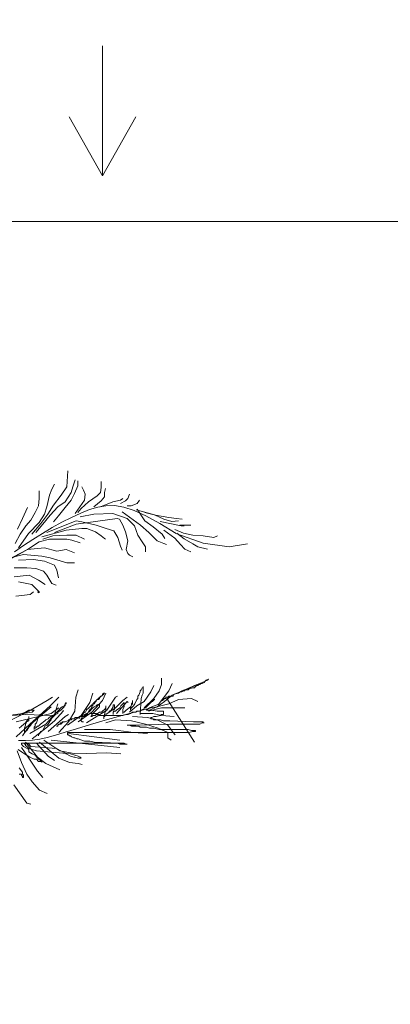
# Model space of a CAD drawing. Units: millimetres. Extents: x 595116 to 630915, y 909473 to 920225.
# Tile 40 of 134: x 629672 to 629682, y 919164 to 919190. Entities that reach past the tile are written whole.
import ezdxf

# ---------------------------------------------------------------- set-up
doc = ezdxf.new("R2010")
doc.units = ezdxf.units.MM
doc.layers.add('Dimension', color=3, linetype='Continuous', lineweight=18)
doc.layers.add('L-PLNT', color=85, linetype='Continuous', lineweight=13)
doc.styles.get("Standard").update_dxf_attribs({"font": 'arial.ttf'})
doc.dimstyles.new('ISO-25', dxfattribs={"dimtxt": 9, "dimasz": 6, "dimexe": 1.25, "dimexo": 0.625, "dimtad": 1, "dimlunit": 4, "dimtxsty": 'Standard', "dimcen": 2.5, "dimadec": 0, "dimazin": 0, "dimtfac": 1, "dimtmove": 0, "dimatfit": 3, "dimfxl": 1, "dimarcsym": 0})

# ---------------------------------------------------------------- blocks, each defined once
blk = doc.blocks.new('A$C4FB75ABC')
for p, q in [((4.1608, 3.5609), (4.1668, 3.6742)), ((4.2026, 3.5609), (4.2205, 3.6086)), ((4.2384, 3.5668), (4.2384, 3.6026)), ((4.4054, 3.5549), (4.4054, 3.5967)), ((3.964, 3.4774), (3.964, 3.5311)), ((4.0356, 3.5013), (4.0535, 3.543)), ((4.0535, 3.543), (4.0714, 3.5788)), ((4.1191, 3.5013), (4.1608, 3.5609)), ((4.1489, 3.4536), (4.1907, 3.5192)), ((4.1907, 3.5192), (4.2026, 3.5609)), ((4.1907, 3.4655), (4.2145, 3.5132)), ((4.2145, 3.5132), (4.2384, 3.5668)), ((4.2801, 3.537), (4.2682, 3.5609)), ((4.2921, 3.5072), (4.2801, 3.537)), ((4.3756, 3.4953), (4.3994, 3.5192)), ((4.3994, 3.5192), (4.4054, 3.5549)), ((4.4293, 3.5192), (4.4352, 3.549)), ((4.4293, 3.4893), (4.4293, 3.5192)), ((3.958, 3.4238), (3.964, 3.4774)), ((4.0177, 3.4178), (4.0356, 3.5013)), ((4.0654, 3.4297), (4.1191, 3.5013)), ((4.0952, 3.4178), (4.1489, 3.4536)), ((4.1489, 3.4118), (4.1907, 3.4655)), ((4.2205, 3.3701), (4.2861, 3.4655)), ((4.2622, 3.4059), (4.3159, 3.4536)), ((4.2861, 3.4655), (4.2921, 3.5072)), ((4.3159, 3.4536), (4.3756, 3.4953)), ((4.3517, 3.4178), (4.4054, 3.4595)), ((4.3994, 3.4178), (4.4889, 3.4536)), ((4.4054, 3.4595), (4.4293, 3.4893)), ((4.4889, 3.4536), (4.5426, 3.4655)), ((4.5426, 3.4655), (4.5605, 3.4774)), ((4.5426, 3.4416), (4.5784, 3.4595)), ((4.5784, 3.4595), (4.5963, 3.4774)), ((4.5963, 3.4774), (4.6082, 3.5072)), ((4.6619, 3.4416), (4.6798, 3.4655)), ((3.8447, 3.3343), (3.8805, 3.4118)), ((3.9044, 3.3224), (3.9342, 3.3761)), ((3.9342, 3.3761), (3.958, 3.4238)), ((3.9998, 3.3641), (4.0177, 3.4178)), ((4.0237, 3.3641), (4.0654, 3.4297)), ((4.0415, 3.3582), (4.0952, 3.4178)), ((4.1012, 3.3522), (4.1489, 3.4118)), ((4.1935, 3.342), (4.2593, 3.3722)), ((4.2384, 3.3761), (4.2622, 3.4059)), ((4.2593, 3.3722), (4.322, 3.3969)), ((4.322, 3.3969), (4.3813, 3.4152)), ((4.3813, 3.4152), (4.4396, 3.4254)), ((4.4396, 3.4254), (4.5001, 3.426)), ((4.5001, 3.426), (4.5657, 3.4153)), ((4.5545, 3.382), (4.6858, 3.2866)), ((4.5657, 3.4153), (4.6395, 3.3917)), ((4.5903, 3.4238), (4.6201, 3.4238)), ((4.6201, 3.4238), (4.6619, 3.4416)), ((4.6395, 3.3917), (4.7247, 3.3534)), ((4.6551, 3.396), (4.7847, 3.3597)), ((4.6619, 3.3999), (4.7156, 3.3164)), ((4.7156, 3.3761), (4.7931, 3.3582)), ((3.8089, 3.2568), (3.8447, 3.3343)), ((3.8686, 3.2807), (3.9044, 3.3224)), ((3.8865, 3.227), (3.964, 3.3045)), ((3.964, 3.3045), (3.9998, 3.3641)), ((3.9759, 3.2986), (4.0237, 3.3641)), ((3.9879, 3.2926), (4.0415, 3.3582)), ((4.0177, 3.233), (4.2265, 3.3164)), ((4.0565, 3.2687), (4.1256, 3.3072)), ((4.0654, 3.3105), (4.1012, 3.3522)), ((4.1256, 3.3072), (4.1935, 3.342)), ((4.2265, 3.2926), (4.5187, 3.3343)), ((4.2265, 3.3164), (4.2682, 3.3105)), ((4.2563, 3.3463), (4.3517, 3.3641)), ((4.2682, 3.3105), (4.3696, 3.2866)), ((4.3517, 3.3641), (4.4889, 3.3701)), ((4.4889, 3.3701), (4.5903, 3.3343)), ((4.5187, 3.3343), (4.5366, 3.3284)), ((4.5366, 3.3284), (4.5605, 3.2866)), ((4.5903, 3.3343), (4.644, 3.2807)), ((4.7156, 3.3164), (4.7752, 3.2747)), ((4.7247, 3.3534), (4.8242, 3.2989)), ((4.7847, 3.3597), (4.8521, 3.3286)), ((4.7931, 3.3582), (4.8886, 3.3403)), ((4.8262, 3.3131), (4.9765, 3.282)), ((4.8521, 3.3286), (4.9091, 3.3131)), ((4.8886, 3.3403), (4.9422, 3.3343)), ((4.9091, 3.3131), (4.9558, 3.3183)), ((4.9422, 3.3343), (4.984, 3.3284)), ((3.8268, 3.2211), (3.8686, 3.2807)), ((3.9103, 3.2211), (3.9759, 3.2986)), ((3.9401, 3.233), (3.9879, 3.2926)), ((3.9819, 3.2032), (4.1549, 3.2509)), ((3.9871, 3.2274), (4.0565, 3.2687)), ((4.0714, 3.233), (4.2265, 3.2926)), ((4.1549, 3.2509), (4.2682, 3.2628)), ((4.2682, 3.2628), (4.304, 3.2628)), ((4.304, 3.2628), (4.3637, 3.2389)), ((4.3637, 3.2389), (4.4054, 3.2091)), ((4.3696, 3.2866), (4.4412, 3.2628)), ((4.4412, 3.2628), (4.4949, 3.2449)), ((4.4949, 3.2449), (4.5247, 3.1972)), ((4.5605, 3.2866), (4.5784, 3.2389)), ((4.5784, 3.2389), (4.5963, 3.1734)), ((4.644, 3.2807), (4.6679, 3.2151)), ((4.6858, 3.2866), (4.7454, 3.233)), ((4.7454, 3.233), (4.8051, 3.1734)), ((4.7752, 3.2747), (4.8408, 3.2211)), ((4.8242, 3.2989), (4.9411, 3.2265)), ((4.8521, 3.2509), (4.9299, 3.1939)), ((4.9299, 3.2561), (4.9921, 3.2302)), ((4.9661, 3.2866), (5.0079, 3.2866)), ((4.9765, 3.282), (4.9973, 3.282)), ((5.0079, 3.2866), (5.0437, 3.2866)), ((3.791, 3.1555), (3.8268, 3.2211)), ((3.8149, 3.1257), (3.8865, 3.227)), ((3.8516, 3.1401), (3.9185, 3.1843)), ((3.8805, 3.1137), (3.964, 3.1674)), ((3.9185, 3.1843), (3.9871, 3.2274)), ((3.964, 3.1674), (4.0356, 3.1853)), ((3.9879, 3.1853), (4.0594, 3.2091)), ((4.0356, 3.1853), (4.1072, 3.1853)), ((4.0594, 3.2091), (4.1608, 3.2151)), ((4.1072, 3.1853), (4.1608, 3.1853)), ((4.1608, 3.2151), (4.2265, 3.2151)), ((4.1608, 3.1853), (4.1966, 3.1793)), ((4.1966, 3.1793), (4.2563, 3.1614)), ((4.2265, 3.2151), (4.2861, 3.1853)), ((4.4054, 3.2091), (4.4293, 3.1912)), ((4.4293, 3.1912), (4.4352, 3.1853)), ((4.5247, 3.1972), (4.5426, 3.1376)), ((4.5963, 3.1734), (4.5844, 3.1137)), ((4.6679, 3.2151), (4.6977, 3.1674)), ((4.6977, 3.1674), (4.7215, 3.1316)), ((4.8051, 3.1734), (4.8528, 3.1555)), ((4.8408, 3.2211), (4.8587, 3.1912)), ((4.9299, 3.1939), (4.9713, 3.1472)), ((4.9454, 3.2302), (4.9973, 3.1887)), ((4.9454, 3.225), (5.1321, 3.1576)), ((4.9921, 3.2302), (5.0595, 3.2146)), ((4.9973, 3.1887), (5.0595, 3.1524)), ((5.0595, 3.2146), (5.1321, 3.2094)), ((5.1321, 3.2094), (5.2099, 3.1991)), ((5.2099, 3.1991), (5.2358, 3.2094)), ((3.7433, 3.0362), (3.8805, 3.1137)), ((3.7791, 3.0601), (3.8805, 3.1137)), ((3.7873, 3.0958), (3.8516, 3.1401)), ((3.8805, 3.1137), (3.9998, 3.1257)), ((3.9998, 3.1257), (4.0893, 3.1018)), ((4.0893, 3.1018), (4.1549, 3.1137)), ((4.1549, 3.1137), (4.2145, 3.0899)), ((4.5426, 3.1376), (4.5545, 3.1078)), ((4.5844, 3.1137), (4.5963, 3.0839)), ((4.7215, 3.1316), (4.7215, 3.0959)), ((4.8528, 3.1555), (4.8707, 3.1495)), ((4.9713, 3.1472), (5.0025, 3.1162)), ((5.0025, 3.1162), (5.0439, 3.0954)), ((5.0595, 3.1524), (5.0958, 3.1317)), ((5.0958, 3.1317), (5.1632, 3.1162)), ((5.1321, 3.1576), (5.3187, 3.1317)), ((5.3187, 3.1317), (5.4484, 3.1524)), ((3.7552, 3.0541), (3.8507, 3.078)), ((3.8149, 3.0362), (3.9222, 3.0422)), ((3.8507, 3.078), (3.9819, 3.066)), ((3.9222, 3.0422), (3.9998, 3.0303)), ((3.9819, 3.066), (4.0415, 3.0541)), ((3.9998, 3.0303), (4.0714, 3.0005)), ((4.0415, 3.0541), (4.1608, 3.0184)), ((4.5963, 3.0839), (4.6082, 3.072)), ((4.6082, 3.072), (4.6321, 3.0601)), ((3.7851, 2.9826), (3.8745, 2.9826)), ((3.8745, 2.9826), (3.9401, 2.9766)), ((3.9401, 2.9766), (3.9938, 2.9587)), ((3.9938, 2.9587), (4.0177, 2.9289)), ((4.0714, 3.0005), (4.0893, 2.9647)), ((4.0893, 2.9647), (4.1012, 2.911)), ((4.1608, 3.0184), (4.2145, 3.0184)), ((3.7851, 2.917), (3.8924, 2.9289)), ((3.8149, 2.8812), (3.9103, 2.8633)), ((3.8924, 2.9289), (3.958, 2.8932)), ((3.958, 2.8932), (4.0058, 2.8633)), ((4.0177, 2.9289), (4.0535, 2.8693)), ((3.9103, 2.8633), (3.964, 2.8097)), ((4.0535, 2.8693), (4.0833, 2.8574)), ((3.797, 2.7799), (3.8984, 2.7918)), ((3.8984, 2.7918), (3.9222, 2.8097)), ((3.964, 2.8037), (3.9521, 2.8097)), ((3.964, 2.8097), (3.964, 2.8037)), ((4.835, 2.1495), (4.835, 2.1952)), ((5.1477, 2.1724), (5.1629, 2.18)), ((5.1553, 2.18), (5.1477, 2.1724)), ((5.1706, 2.1876), (5.1553, 2.18)), ((5.1629, 2.18), (5.1706, 2.1876)), ((4.2249, 2.058), (4.2402, 2.1114)), ((4.6825, 2.1038), (4.6901, 2.1114)), ((4.6901, 2.1114), (4.6977, 2.1266)), ((4.6977, 2.1266), (4.7054, 2.1266)), ((4.7054, 2.1266), (4.7054, 2.1343)), ((4.7054, 2.1343), (4.7054, 2.0885)), ((4.7587, 2.0961), (4.7816, 2.1419)), ((4.8198, 2.1038), (4.835, 2.1495)), ((4.8884, 2.1038), (4.9113, 2.1571)), ((4.9113, 2.0733), (5.079, 2.1419)), ((5.018, 2.119), (4.9799, 2.1038)), ((5.0028, 2.1038), (5.0028, 2.1114)), ((5.0028, 2.1114), (5.0257, 2.1114)), ((5.0333, 2.1266), (5.018, 2.119)), ((5.0257, 2.1114), (5.0333, 2.119)), ((5.0562, 2.1343), (5.0333, 2.1266)), ((5.0333, 2.119), (5.0562, 2.1266)), ((5.0714, 2.1419), (5.0562, 2.1343)), ((5.0562, 2.1266), (5.0714, 2.1266)), ((5.1095, 2.1571), (5.0714, 2.1419)), ((5.0714, 2.1266), (5.079, 2.1343)), ((5.079, 2.1343), (5.0867, 2.1419)), ((5.0867, 2.1419), (5.0943, 2.1419)), ((5.0943, 2.1419), (5.1019, 2.1495)), ((5.1019, 2.1495), (5.1095, 2.1495)), ((5.1248, 2.1648), (5.1095, 2.1571)), ((5.1095, 2.1495), (5.1172, 2.1571)), ((5.1172, 2.1571), (5.1248, 2.1571)), ((5.1477, 2.1724), (5.1248, 2.1648)), ((5.1248, 2.1571), (5.1401, 2.1648)), ((5.1401, 2.1648), (5.1477, 2.1724)), ((4.019, 2.0352), (4.0571, 2.058)), ((4.0419, 1.9971), (4.1029, 2.058)), ((4.2173, 1.9589), (4.2249, 2.058)), ((4.324, 2.0199), (4.3469, 2.0885)), ((4.3698, 2.0352), (4.3774, 2.0428)), ((4.3774, 2.0428), (4.3698, 2.0352)), ((4.3851, 2.0504), (4.3774, 2.0428)), ((4.3774, 2.0428), (4.3851, 2.0428)), ((4.3927, 2.058), (4.3851, 2.0504)), ((4.3851, 2.0428), (4.3927, 2.0504)), ((4.4079, 2.0657), (4.3927, 2.058)), ((4.3927, 2.0504), (4.3927, 2.058)), ((4.3927, 2.058), (4.4003, 2.058)), ((4.4003, 2.058), (4.4003, 2.0657)), ((4.4003, 2.0657), (4.4079, 2.0657)), ((4.4079, 2.0657), (4.4156, 2.0733)), ((4.4156, 2.0733), (4.4079, 2.0657)), ((4.4156, 2.0809), (4.4232, 2.0885)), ((4.4156, 2.0352), (4.4384, 2.0885)), ((4.4156, 2.0733), (4.4156, 2.0809)), ((4.4232, 2.0809), (4.4156, 2.0733)), ((4.4232, 2.0885), (4.4308, 2.0885)), ((4.4308, 2.0885), (4.4232, 2.0885)), ((4.4232, 2.0885), (4.4232, 2.0809)), ((4.4461, 1.9666), (4.5071, 2.058)), ((4.5071, 2.058), (4.5223, 2.0657)), ((4.5605, 2.0352), (4.591, 2.058)), ((4.6444, 2.0123), (4.6596, 2.0428)), ((4.6596, 2.0428), (4.6672, 2.0504)), ((4.6672, 2.0657), (4.6749, 2.0733)), ((4.6672, 2.0504), (4.6672, 2.0657)), ((4.6749, 2.0733), (4.6825, 2.0961)), ((4.6825, 2.0961), (4.6825, 2.1038)), ((4.6901, 2.0504), (4.6825, 1.9361)), ((4.6977, 2.0733), (4.6901, 2.0504)), ((4.7054, 2.0885), (4.6977, 2.0733)), ((4.713, 2.0275), (4.7587, 2.0961)), ((4.713, 1.9818), (4.7816, 2.0504)), ((4.7816, 2.0504), (4.8198, 2.1038)), ((4.7892, 2.0428), (4.7816, 2.0428)), ((4.7816, 2.0428), (4.7816, 2.0352)), ((4.8121, 2.0047), (4.8884, 2.1038)), ((4.8426, 2.0352), (4.8579, 2.0504)), ((4.8579, 2.0275), (4.9113, 2.0733)), ((4.8579, 2.0504), (4.8655, 2.0504)), ((4.8655, 2.0504), (4.8655, 2.058)), ((4.8655, 2.058), (4.8808, 2.058)), ((4.8808, 2.0504), (4.8731, 2.0504)), ((4.8731, 2.0504), (5.0714, 1.7379)), ((4.8808, 2.058), (4.8884, 2.0657)), ((4.896, 2.058), (4.8808, 2.058)), ((4.8808, 2.058), (4.8808, 2.0504)), ((4.8884, 2.0657), (4.9036, 2.0657)), ((4.8884, 2.0123), (4.957, 2.0428)), ((4.9036, 2.0657), (4.896, 2.058)), ((4.9036, 2.0657), (4.9113, 2.0733)), ((4.9189, 2.0657), (4.9036, 2.0657)), ((4.9113, 2.0733), (4.9265, 2.0809)), ((4.9265, 2.0809), (4.9189, 2.0657)), ((4.9265, 2.0809), (4.957, 2.0885)), ((4.9494, 2.0885), (4.9265, 2.0809)), ((4.9799, 2.1038), (4.9494, 2.0885)), ((4.957, 2.0885), (4.9723, 2.0961)), ((4.957, 2.0428), (5.0485, 2.0504)), ((4.9723, 2.0961), (4.9799, 2.0961)), ((4.9799, 2.0961), (4.9952, 2.1038)), ((4.9952, 2.1038), (5.0028, 2.1038)), ((5.0485, 2.0504), (5.0943, 2.0275)), ((3.8894, 1.9589), (4.019, 2.0352)), ((3.958, 1.9132), (4.0495, 1.9894)), ((3.9656, 1.9285), (4.0419, 1.9971)), ((4.0495, 1.9437), (4.1029, 1.9818)), ((4.0724, 1.9361), (4.0953, 2.0123)), ((4.1181, 1.9818), (4.1029, 1.9666)), ((4.1258, 1.9894), (4.1181, 1.9818)), ((4.1181, 1.9666), (4.1334, 1.9818)), ((4.141, 1.9971), (4.1258, 1.9894)), ((4.1334, 1.9818), (4.141, 1.9894)), ((4.1486, 2.0123), (4.141, 1.9971)), ((4.141, 1.9894), (4.141, 1.9971)), ((4.141, 1.9971), (4.1486, 1.9971)), ((4.1563, 2.0199), (4.1486, 2.0123)), ((4.1486, 1.9971), (4.1486, 2.0123)), ((4.1486, 2.0123), (4.1563, 2.0123)), ((4.1563, 2.0123), (4.1563, 2.0199)), ((4.263, 1.9285), (4.324, 2.0199)), ((4.3088, 1.9742), (4.3012, 1.9742)), ((4.3012, 1.9742), (4.3012, 1.9666)), ((4.3164, 1.9818), (4.3088, 1.9742)), ((4.3317, 1.9971), (4.3164, 1.9818)), ((4.3164, 1.9513), (4.3469, 1.9818)), ((4.324, 1.9666), (4.324, 1.9742)), ((4.324, 1.9742), (4.3317, 1.9742)), ((4.3393, 2.0047), (4.3317, 1.9971)), ((4.3317, 1.9742), (4.3393, 1.9894)), ((4.3393, 1.9513), (4.4156, 2.0352)), ((4.3546, 2.0123), (4.3393, 2.0047)), ((4.3393, 1.9894), (4.3393, 1.9971)), ((4.3393, 1.9971), (4.3469, 1.9971)), ((4.3469, 2.0123), (4.3622, 2.0275)), ((4.3469, 1.9971), (4.3469, 2.0123)), ((4.3469, 1.9818), (4.3546, 1.9894)), ((4.3698, 2.0352), (4.3546, 2.0123)), ((4.3546, 1.9894), (4.3698, 1.9971)), ((4.3622, 2.0275), (4.3698, 2.0275)), ((4.3698, 2.0275), (4.3698, 2.0352)), ((4.3698, 1.9971), (4.3774, 2.0047)), ((4.3851, 1.9818), (4.3698, 1.9666)), ((4.3774, 2.0047), (4.3927, 2.0123)), ((4.3927, 1.9894), (4.3851, 1.9818)), ((4.3927, 2.0123), (4.3927, 1.9894)), ((4.4156, 1.9589), (4.4308, 1.9742)), ((4.4308, 1.9742), (4.4384, 1.9818)), ((4.4384, 1.9818), (4.4384, 1.9971)), ((4.4384, 1.9971), (4.4384, 1.9589)), ((4.4384, 1.9361), (4.5071, 1.9818)), ((4.4766, 1.9666), (4.4918, 1.9894)), ((4.4918, 1.9894), (4.4918, 2.0047)), ((4.4918, 2.0047), (4.4995, 2.0047)), ((4.4995, 1.9742), (4.4918, 1.9513)), ((4.4995, 2.0047), (4.4995, 1.9742)), ((4.5071, 1.9818), (4.5605, 2.0352)), ((4.5147, 1.9437), (4.591, 2.0275)), ((4.5147, 1.9666), (4.5376, 1.9818)), ((4.5376, 1.9818), (4.5452, 1.9971)), ((4.5452, 1.9971), (4.5528, 2.0047)), ((4.5528, 2.0047), (4.5605, 2.0123)), ((4.5605, 2.0123), (4.5681, 2.0199)), ((4.5681, 1.9894), (4.5605, 1.9742)), ((4.5605, 1.9742), (4.5605, 1.9437)), ((4.5681, 2.0199), (4.5681, 1.9894)), ((4.5833, 1.9666), (4.6138, 1.9894)), ((4.591, 2.0275), (4.5986, 2.0199)), ((4.7725, 1.9851), (4.5975, 1.9398)), ((4.6062, 1.9513), (4.6596, 1.9971)), ((4.6138, 1.9894), (4.6215, 2.0047)), ((4.6215, 2.0047), (4.6138, 1.9818)), ((4.6138, 1.9818), (4.6138, 1.9666)), ((4.6138, 1.9742), (4.6215, 1.9818)), ((4.6138, 1.9666), (4.6138, 1.9742)), ((4.6215, 2.0123), (4.6291, 2.0199)), ((4.6215, 2.0047), (4.6215, 2.0123)), ((4.6291, 2.0123), (4.6215, 2.0047)), ((4.6215, 1.9818), (4.6367, 1.9971)), ((4.6291, 2.0199), (4.6291, 2.0352)), ((4.6291, 2.0352), (4.6291, 2.0123)), ((4.6367, 1.9971), (4.6444, 2.0123)), ((4.6596, 1.9971), (4.713, 2.0275)), ((4.7054, 1.9742), (4.6901, 1.9666)), ((4.7206, 1.9818), (4.7054, 1.9742)), ((4.7359, 1.9971), (4.7206, 1.9818)), ((4.7282, 1.9666), (4.7282, 1.9742)), ((4.7282, 1.9742), (4.7359, 1.9742)), ((4.7435, 2.0047), (4.7359, 1.9971)), ((4.7359, 1.9742), (4.7511, 1.9818)), ((4.7511, 2.0123), (4.7435, 2.0047)), ((4.7435, 1.9589), (4.835, 1.9818)), ((4.7664, 2.0275), (4.7511, 2.0123)), ((4.7511, 1.9818), (4.7664, 1.9894)), ((4.7511, 1.9666), (4.8045, 1.9894)), ((4.774, 2.0275), (4.7664, 2.0275)), ((4.7664, 1.9894), (4.8045, 2.0047)), ((4.7816, 2.0352), (4.774, 2.0352)), ((4.774, 2.0352), (4.774, 2.0275)), ((4.774, 1.9818), (4.8884, 2.0123)), ((4.8045, 1.9894), (4.8579, 2.0275)), ((4.8045, 2.0047), (4.8198, 2.0123)), ((4.8198, 2.0123), (4.8274, 2.0275)), ((4.8274, 2.0275), (4.8426, 2.0352)), ((4.835, 1.9818), (4.9494, 1.9818)), ((4.9494, 1.9818), (5.0028, 1.9818)), ((3.5843, 1.9132), (3.8665, 1.9361)), ((3.7445, 1.9285), (3.9122, 1.9513)), ((3.7521, 1.8903), (3.8894, 1.9589)), ((3.7978, 1.8827), (4.0495, 1.9437)), ((3.8665, 1.9513), (3.8207, 1.9361)), ((3.8894, 1.9666), (3.8665, 1.9513)), ((3.8665, 1.9361), (4.0495, 1.9285)), ((3.8894, 1.9056), (3.8741, 1.8903)), ((3.9275, 1.9666), (3.8894, 1.9666)), ((3.8894, 1.8903), (3.8894, 1.9208)), ((3.8894, 1.9208), (3.8894, 1.9056)), ((3.897, 1.8675), (3.9656, 1.9285)), ((3.897, 1.8599), (3.958, 1.9132)), ((3.9122, 1.9513), (3.9199, 1.9589)), ((3.9351, 1.898), (3.9122, 1.8751)), ((3.9199, 1.9589), (3.9275, 1.9666)), ((3.9504, 1.9056), (3.9351, 1.898)), ((3.9427, 1.8751), (3.9504, 1.898)), ((3.958, 1.9208), (3.9504, 1.9056)), ((3.9504, 1.9056), (3.958, 1.9132)), ((3.9504, 1.898), (3.9504, 1.9056)), ((3.958, 1.9208), (3.9656, 1.9285)), ((3.9656, 1.9285), (3.958, 1.9208)), ((3.958, 1.9132), (3.958, 1.9208)), ((3.9656, 1.9285), (3.9656, 1.9361)), ((3.9656, 1.9361), (3.9656, 1.9285)), ((4.0114, 1.898), (4.0037, 1.8903)), ((4.0114, 1.8675), (4.0724, 1.9361)), ((4.0266, 1.9056), (4.0114, 1.898)), ((4.0266, 1.8141), (4.1486, 1.9208)), ((4.0343, 1.9132), (4.0266, 1.9056)), ((4.0571, 1.9285), (4.0343, 1.9132)), ((4.0419, 1.8903), (4.0495, 1.898)), ((4.0495, 1.9056), (4.0571, 1.9132)), ((4.0495, 1.898), (4.0495, 1.9056)), ((4.0724, 1.9361), (4.0571, 1.9285)), ((4.0571, 1.9132), (4.0724, 1.9285)), ((4.0724, 1.8903), (4.1334, 1.9589)), ((4.08, 1.9437), (4.0724, 1.9361)), ((4.0724, 1.9285), (4.08, 1.9361)), ((4.1029, 1.9666), (4.08, 1.9437)), ((4.08, 1.9361), (4.0953, 1.9437)), ((4.0953, 1.9513), (4.1181, 1.9666)), ((4.0953, 1.9437), (4.0953, 1.9513)), ((4.1334, 1.9589), (4.1334, 1.9666)), ((4.1486, 1.9208), (4.1715, 1.9361)), ((4.1639, 1.8599), (4.263, 1.9285)), ((4.1715, 1.8827), (4.2173, 1.9589)), ((4.1944, 1.898), (4.1715, 1.898)), ((4.1715, 1.898), (4.1715, 1.8903)), ((4.2173, 1.9056), (4.1944, 1.9056)), ((4.1944, 1.9056), (4.1944, 1.898)), ((4.2478, 1.9132), (4.2173, 1.9132)), ((4.2173, 1.9132), (4.2173, 1.9056)), ((4.2402, 1.8827), (4.3393, 1.9513)), ((4.2554, 1.9208), (4.2478, 1.9132)), ((4.2478, 1.9056), (4.2478, 1.9208)), ((4.2478, 1.9208), (4.263, 1.9208)), ((4.263, 1.9208), (4.2478, 1.9132)), ((4.2478, 1.9132), (4.2478, 1.9056)), ((4.263, 1.9208), (4.2554, 1.9208)), ((4.2707, 1.9361), (4.263, 1.9285)), ((4.263, 1.9285), (4.263, 1.9208)), ((4.263, 1.9208), (4.2707, 1.9285)), ((4.2859, 1.9208), (4.263, 1.9208)), ((4.263, 1.9056), (4.2707, 1.9132)), ((4.263, 1.8903), (4.263, 1.9056)), ((4.2859, 1.9513), (4.2707, 1.9361)), ((4.2707, 1.9285), (4.3012, 1.9437)), ((4.2707, 1.9208), (4.2859, 1.9285)), ((4.2707, 1.9132), (4.2707, 1.9208)), ((4.2935, 1.9513), (4.2859, 1.9513)), ((4.2859, 1.9285), (4.2935, 1.9361)), ((4.2935, 1.9285), (4.2859, 1.9208)), ((4.3012, 1.9666), (4.2935, 1.9513)), ((4.2935, 1.9361), (4.3012, 1.9361)), ((4.3012, 1.9285), (4.2935, 1.9285)), ((4.3012, 1.8751), (4.4461, 1.9666)), ((4.3012, 1.9437), (4.3164, 1.9513)), ((4.3012, 1.9361), (4.3088, 1.9437)), ((4.3088, 1.9361), (4.3012, 1.9285)), ((4.3088, 1.9437), (4.3164, 1.9589)), ((4.3317, 1.9437), (4.3088, 1.9361)), ((4.3164, 1.9589), (4.324, 1.9666)), ((4.4513, 1.8996), (4.3302, 1.8644)), ((4.3698, 1.9437), (4.3317, 1.9437)), ((4.3393, 1.9361), (4.3317, 1.9208)), ((4.3317, 1.9208), (4.3393, 1.9208)), ((4.3469, 1.9437), (4.3393, 1.9361)), ((4.3393, 1.9208), (4.3469, 1.9285)), ((4.3622, 1.9589), (4.3469, 1.9437)), ((4.3469, 1.9285), (4.3622, 1.9285)), ((4.3698, 1.9666), (4.3622, 1.9589)), ((4.3622, 1.9285), (4.3698, 1.9361)), ((4.3698, 1.9361), (4.3927, 1.9513)), ((4.3774, 1.9361), (4.3698, 1.9437)), ((4.3851, 1.9361), (4.3774, 1.9361)), ((4.3927, 1.9285), (4.3851, 1.9361)), ((4.3927, 1.9513), (4.4079, 1.9513)), ((4.5605, 1.9285), (4.3927, 1.9285)), ((4.4079, 1.9513), (4.4156, 1.9589)), ((4.4308, 1.9437), (4.4232, 1.9208)), ((4.4232, 1.9208), (4.4232, 1.9056)), ((4.4232, 1.9056), (4.4232, 1.9208)), ((4.4232, 1.9208), (4.4308, 1.9208)), ((4.4384, 1.9589), (4.4308, 1.9513)), ((4.4308, 1.9513), (4.4308, 1.9437)), ((4.4308, 1.9208), (4.4384, 1.9361)), ((4.4384, 1.9361), (4.4613, 1.9513)), ((4.4384, 1.8751), (4.5071, 1.898)), ((4.5975, 1.9398), (4.4513, 1.8996)), ((4.4613, 1.9589), (4.4766, 1.9666)), ((4.4613, 1.9513), (4.4613, 1.9589)), ((4.4918, 1.9513), (4.5071, 1.9589)), ((4.4918, 1.9513), (4.4918, 1.9361)), ((4.4918, 1.9361), (4.4918, 1.9513)), ((4.5071, 1.9589), (4.5147, 1.9666)), ((4.5071, 1.898), (4.6215, 1.8903)), ((4.5605, 1.9513), (4.5681, 1.9513)), ((4.5605, 1.9437), (4.5605, 1.9513)), ((4.5833, 1.9361), (4.5605, 1.9285)), ((4.5681, 1.9513), (4.5757, 1.9589)), ((4.5757, 1.9589), (4.5833, 1.9666)), ((4.5986, 1.9361), (4.5833, 1.9361)), ((4.6138, 1.9437), (4.5986, 1.9361)), ((4.6291, 1.9513), (4.6138, 1.9437)), ((4.652, 1.9513), (4.6291, 1.9513)), ((4.6291, 1.9208), (4.7359, 1.9132)), ((4.6596, 1.9589), (4.652, 1.9513)), ((4.6825, 1.9589), (4.6596, 1.9589)), ((4.6901, 1.9666), (4.6825, 1.9589)), ((4.6825, 1.9437), (4.774, 1.9437)), ((4.7587, 1.9666), (4.7282, 1.9666)), ((4.7359, 1.9132), (4.8045, 1.898)), ((4.8045, 1.9589), (4.7587, 1.9666)), ((4.7587, 1.9056), (4.7587, 1.9132)), ((4.7587, 1.9132), (4.7664, 1.9132)), ((4.774, 1.9056), (4.7587, 1.9056)), ((4.7664, 1.9132), (4.7816, 1.9208)), ((4.774, 1.9437), (4.835, 1.9285)), ((4.7816, 1.898), (4.774, 1.9056)), ((4.7816, 1.9208), (4.7969, 1.9208)), ((4.8274, 1.898), (4.7816, 1.898)), ((4.7969, 1.9208), (4.8274, 1.9285)), ((4.8503, 1.9589), (4.8045, 1.9589)), ((4.8045, 1.898), (4.8808, 1.8599)), ((4.8274, 1.9285), (4.835, 1.9361)), ((4.8503, 1.8903), (4.8274, 1.898)), ((4.835, 1.9361), (4.8503, 1.9361)), ((4.835, 1.9285), (4.9265, 1.9208)), ((4.8503, 1.9361), (4.8503, 1.9589)), ((3.7978, 1.776), (3.897, 1.8675)), ((3.836, 1.8522), (3.8207, 1.837)), ((3.8665, 1.8751), (3.836, 1.8522)), ((3.8436, 1.7836), (3.897, 1.8599)), ((3.8589, 1.837), (3.8665, 1.8599)), ((3.8589, 1.8065), (3.8589, 1.837)), ((3.8741, 1.8903), (3.8665, 1.8751)), ((3.8665, 1.8675), (3.8741, 1.8827)), ((3.8665, 1.8599), (3.8665, 1.8675)), ((3.8741, 1.8827), (3.8894, 1.8903)), ((3.8894, 1.8446), (3.8741, 1.8217)), ((3.9046, 1.8599), (3.8894, 1.8446)), ((3.897, 1.7989), (4.0114, 1.8675)), ((3.9122, 1.8751), (3.9046, 1.8599)), ((3.9122, 1.7608), (4.0114, 1.837)), ((3.9275, 1.8446), (3.9351, 1.8522)), ((3.9275, 1.8294), (3.9275, 1.8446)), ((3.9351, 1.837), (3.9275, 1.837)), ((3.9275, 1.837), (3.9275, 1.8294)), ((3.9351, 1.8675), (3.9427, 1.8751)), ((3.9351, 1.8522), (3.9351, 1.8675)), ((3.9427, 1.8446), (3.9351, 1.837)), ((3.9504, 1.8522), (3.9427, 1.8446)), ((3.958, 1.8522), (3.9504, 1.8522)), ((3.9656, 1.8599), (3.958, 1.8522)), ((3.9732, 1.8675), (3.9656, 1.8599)), ((4.0037, 1.8903), (3.9732, 1.8675)), ((3.9885, 1.8217), (4.0037, 1.8522)), ((4.0037, 1.8522), (4.019, 1.8599)), ((4.0114, 1.837), (4.0724, 1.8903)), ((4.019, 1.8599), (4.0266, 1.8675)), ((4.0266, 1.8675), (4.0419, 1.8903)), ((4.0953, 1.8522), (4.0876, 1.8522)), ((4.0876, 1.8522), (4.0953, 1.8522)), ((4.1029, 1.8675), (4.0953, 1.8599)), ((4.0953, 1.8599), (4.1105, 1.8675)), ((4.0953, 1.8599), (4.0953, 1.8522)), ((4.0953, 1.8522), (4.0953, 1.8599)), ((4.1029, 1.8065), (4.1715, 1.8827)), ((4.1105, 1.8675), (4.1029, 1.8675)), ((4.1181, 1.8751), (4.1105, 1.8675)), ((4.1105, 1.8675), (4.1181, 1.8675)), ((4.1258, 1.8751), (4.1181, 1.8751)), ((4.1181, 1.8675), (4.1258, 1.8751)), ((4.1334, 1.8827), (4.1258, 1.8751)), ((4.1258, 1.8751), (4.1258, 1.8827)), ((4.1258, 1.8827), (4.1334, 1.8827)), ((4.1486, 1.8827), (4.1334, 1.8827)), ((4.2303, 1.8341), (4.1477, 1.8087)), ((4.1639, 1.8903), (4.1486, 1.8827)), ((4.1715, 1.8903), (4.1639, 1.8903)), ((4.3302, 1.8644), (4.2303, 1.8341)), ((4.2707, 1.8827), (4.263, 1.8903)), ((4.2783, 1.8827), (4.2707, 1.8827)), ((4.2859, 1.8294), (4.4689, 1.8294)), ((4.4689, 1.8294), (4.53, 1.8217)), ((4.6062, 1.8599), (4.591, 1.8599)), ((4.591, 1.8599), (4.652, 1.8599)), ((4.6215, 1.8522), (4.6062, 1.8599)), ((4.6215, 1.8903), (4.7206, 1.8675)), ((4.6749, 1.8522), (4.6215, 1.8522)), ((4.652, 1.8599), (4.896, 1.8675)), ((4.6825, 1.8446), (4.6749, 1.8522)), ((4.7282, 1.8446), (4.6825, 1.8446)), ((4.7206, 1.8675), (4.8121, 1.837)), ((4.7511, 1.837), (4.7282, 1.8446)), ((4.7816, 1.837), (4.7511, 1.837)), ((4.8198, 1.8294), (4.7816, 1.837)), ((4.8121, 1.837), (4.8808, 1.8065)), ((5.0257, 1.8294), (4.8198, 1.8294)), ((4.896, 1.8903), (4.8503, 1.8903)), ((4.8808, 1.8599), (4.9189, 1.8065)), ((5.0638, 1.8827), (4.896, 1.8903)), ((4.896, 1.8675), (5.1095, 1.8675)), ((5.0485, 1.8217), (5.0257, 1.8294)), ((5.1324, 1.8827), (5.0638, 1.8827)), ((5.1095, 1.8675), (5.1248, 1.8751)), ((5.1248, 1.8751), (5.1401, 1.8751)), ((5.1324, 1.8751), (5.1324, 1.8827)), ((5.1401, 1.8751), (5.1324, 1.8751)), ((3.8665, 1.8141), (3.8589, 1.8065)), ((3.8741, 1.8217), (3.8665, 1.8141)), ((3.9666, 1.7597), (3.916, 1.7521)), ((3.958, 1.7913), (3.9656, 1.7989)), ((3.958, 1.7836), (3.958, 1.7913)), ((3.9656, 1.7989), (3.9732, 1.8065)), ((4.0197, 1.7715), (3.9666, 1.7597)), ((3.9732, 1.8141), (3.9885, 1.8217)), ((3.9732, 1.8065), (3.9732, 1.8141)), ((4.0788, 1.7878), (4.0197, 1.7715)), ((4.1477, 1.8087), (4.0788, 1.7878)), ((4.1639, 1.7913), (4.1639, 1.8065)), ((4.1639, 1.8065), (5.0333, 1.8065)), ((4.1715, 1.7913), (4.1639, 1.7913)), ((4.1715, 1.7989), (4.5376, 1.7531)), ((4.1792, 1.7836), (4.1715, 1.7913)), ((4.1868, 1.7836), (4.1792, 1.7836)), ((4.1944, 1.776), (4.1868, 1.7836)), ((4.2097, 1.7684), (4.1944, 1.776)), ((4.2173, 1.7684), (4.2097, 1.7684)), ((4.2325, 1.7608), (4.2173, 1.7684)), ((4.2402, 1.7608), (4.2325, 1.7608)), ((4.2859, 1.7455), (4.2402, 1.7608)), ((4.53, 1.8217), (4.6367, 1.8065)), ((4.6367, 1.8065), (4.7359, 1.7989)), ((4.8808, 1.8065), (4.8808, 1.7684)), ((4.8808, 1.7684), (4.9036, 1.7531)), ((4.9189, 1.8065), (4.9341, 1.7913)), ((5.0333, 1.8065), (5.0562, 1.8141)), ((5.079, 1.8217), (5.0485, 1.8217)), ((5.0562, 1.8141), (5.079, 1.8141)), ((5.079, 1.8141), (5.079, 1.8217)), ((3.8664, 1.749), (3.8165, 1.7504)), ((3.836, 1.7227), (3.836, 1.7303)), ((3.836, 1.7303), (3.8665, 1.7303)), ((3.8436, 1.715), (3.836, 1.7227)), ((3.836, 1.6998), (3.8894, 1.6236)), ((3.8512, 1.7074), (3.8436, 1.715)), ((3.8894, 1.6845), (3.8512, 1.7074)), ((3.8589, 1.7227), (3.8589, 1.7303)), ((3.8589, 1.7303), (4.5223, 1.7303)), ((3.8665, 1.7227), (3.8589, 1.7227)), ((3.916, 1.7521), (3.8664, 1.749)), ((3.8665, 1.7379), (3.9504, 1.6312)), ((3.8665, 1.7303), (3.8894, 1.7227)), ((3.8665, 1.715), (3.8665, 1.7227)), ((3.8741, 1.7074), (3.8665, 1.715)), ((3.8894, 1.6922), (3.8741, 1.7074)), ((3.8894, 1.7227), (3.9046, 1.7074)), ((3.9122, 1.6845), (3.8894, 1.6922)), ((3.9046, 1.7074), (4.0876, 1.6922)), ((3.9427, 1.7303), (4.0266, 1.6388)), ((3.9656, 1.7379), (4.0495, 1.6693)), ((3.9961, 1.7531), (4.1105, 1.6769)), ((4.0495, 1.7531), (4.5376, 1.6998)), ((4.0876, 1.6922), (4.1181, 1.6769)), ((4.324, 1.7455), (4.2859, 1.7455)), ((4.3546, 1.7379), (4.324, 1.7455)), ((4.53, 1.7303), (4.3546, 1.7379)), ((4.5223, 1.7303), (4.5376, 1.7227)), ((4.5681, 1.7303), (4.53, 1.7303)), ((4.5376, 1.7227), (4.591, 1.7227)), ((4.5833, 1.7227), (4.5681, 1.7303)), ((4.591, 1.7227), (4.5833, 1.7227)), ((3.8055, 1.6769), (3.836, 1.5931)), ((3.8131, 1.6845), (3.836, 1.6693)), ((3.836, 1.6693), (3.8589, 1.6541)), ((3.8589, 1.6541), (3.897, 1.6312)), ((3.8894, 1.6693), (3.8894, 1.6845)), ((3.9122, 1.6541), (3.8894, 1.6693)), ((3.8894, 1.6236), (3.9504, 1.5321)), ((3.897, 1.6312), (3.9275, 1.6159)), ((3.9427, 1.6769), (3.9122, 1.6845)), ((3.9351, 1.6464), (3.9122, 1.6541)), ((3.9275, 1.6159), (3.9427, 1.6159)), ((3.958, 1.6159), (3.9351, 1.6464)), ((4.1868, 1.6541), (3.9427, 1.6769)), ((3.9427, 1.6159), (3.958, 1.6007)), ((3.9504, 1.6312), (4.0114, 1.5855)), ((3.9732, 1.6083), (3.958, 1.6159)), ((4.0266, 1.6388), (4.0724, 1.6083)), ((4.0495, 1.6693), (4.1029, 1.6236)), ((4.1029, 1.6236), (4.1792, 1.5931)), ((4.1105, 1.6769), (4.2249, 1.6541)), ((4.1181, 1.6769), (4.1334, 1.6693)), ((4.1334, 1.6693), (4.1563, 1.6541)), ((4.1563, 1.6541), (4.1868, 1.6388)), ((4.2173, 1.6464), (4.1868, 1.6541)), ((4.1868, 1.6388), (4.2097, 1.6312)), ((4.2097, 1.6312), (4.2173, 1.6312)), ((4.2402, 1.6388), (4.2173, 1.6464)), ((4.2173, 1.6312), (4.2402, 1.6236)), ((4.2249, 1.6541), (4.4461, 1.6617)), ((4.2554, 1.6312), (4.2402, 1.6388)), ((4.2402, 1.6236), (4.263, 1.6236)), ((4.263, 1.6236), (4.2554, 1.6312)), ((4.4461, 1.6617), (4.5452, 1.6541)), ((3.8436, 1.5245), (3.8207, 1.555)), ((3.836, 1.5931), (3.8741, 1.5092)), ((3.958, 1.6007), (3.9809, 1.6007)), ((3.9809, 1.6083), (3.9732, 1.6083)), ((3.9809, 1.5931), (3.9809, 1.6083)), ((3.9809, 1.6007), (3.9809, 1.5931)), ((4.0114, 1.5855), (4.1105, 1.5397)), ((4.1792, 1.5931), (4.2402, 1.5855)), ((4.2402, 1.5855), (4.2707, 1.5778)), ((3.8207, 1.5092), (3.836, 1.5092)), ((3.836, 1.5092), (3.836, 1.5016)), ((3.836, 1.5016), (3.8436, 1.494)), ((3.8436, 1.5092), (3.8436, 1.5245)), ((3.8512, 1.5016), (3.8436, 1.5092)), ((3.8436, 1.494), (3.8436, 1.4864)), ((3.8436, 1.4864), (3.8512, 1.4864)), ((3.8512, 1.4864), (3.8512, 1.5016)), ((3.8741, 1.5092), (3.9122, 1.4559)), ((3.9504, 1.5321), (3.9885, 1.4864)), ((3.7826, 1.433), (3.8741, 1.3034)), ((3.9122, 1.4559), (3.9656, 1.3949)), ((3.9656, 1.3949), (4.019, 1.372)), ((3.8741, 1.3034), (3.9046, 1.2958))]:
    blk.add_line(p, q)
blk = doc.blocks.new('LAWN-GRASS-TUFT')
blk.add_line((0.892, 3.485), (0.892, 0))
blk.add_lwpolyline([(0, 1.577), (0.892, 0), (1.785, 1.577)])
blk = doc.blocks.new('*D216')
at = {"layer": 'Defpoints', "color": 0, "transparency": 16777216}
for p in [(629505.041, 919411.828), (629743.541, 919411.928), (629743.541, 918832.378)]:
    blk.add_point(p, dxfattribs=at)
at = {"layer": 'Dimension', "color": 0, "lineweight": -2, "transparency": 16777216}
for p, q in [((629743.541, 919411.303), (629743.541, 918831.128)), ((629505.041, 919411.203), (629505.041, 918831.128)), ((629511.041, 918832.378), (629737.541, 918832.378))]:
    blk.add_line(p, q, dxfattribs=at)
at = {"layer": 'Dimension', "color": 0, "transparency": 16777216}
for points in [[(629511.041, 918833.378), (629511.041, 918831.378), (629505.041, 918832.378)], [(629737.541, 918833.378), (629737.541, 918831.378), (629743.541, 918832.378)]]:
    blk.add_solid(points, dxfattribs=at)
at = {"layer": 'Dimension', "color": 0, "transparency": 16777216, "insert": (629624.291, 918837.656), "char_height": 9, "attachment_point": 5}
blk.add_mtext('19\'-10 1/2"', dxfattribs=at)

msp = doc.modelspace()

# ---------------------------------------------------------------- linework, layer by layer
at = {"layer": 'L-PLNT'}
msp.add_line((629535.274, 919184.917), (629800.951, 919184.917), dxfattribs=at)

# ---------------------------------------------------------------- block references
msp.add_blockref('LAWN-GRASS-TUFT', (629673.303, 919186.14), dxfattribs=at)
at = {"layer": 'L-PLNT', "xscale": 3.753413438031968, "yscale": 3.753413438031968, "zscale": 3.753413438031968}
msp.add_blockref('A$C4FB75ABC', (629657.627, 919164.449), dxfattribs=at)

# ---------------------------------------------------------------- dimensions: what is measured, and where the dimension line sits
at = {"layer": 'Dimension'}
dim = msp.add_linear_dim(base=(629743.541, 918832.378), p1=(629505.041, 919411.828), p2=(629743.541, 919411.928), dimstyle='ISO-25', override={"dimdec": 1, "dimlfac": 1, "dimrnd": 0, "dimzin": 1, "dimdsep": 46, "dimlunit": 4, "dimfrac": 2}, dxfattribs=at)
dim.commit()
dim.dimension.update_dxf_attribs({"geometry": '*D216', "text_midpoint": (629624.291, 918837.656)})

doc.saveas('drawing.dxf')
